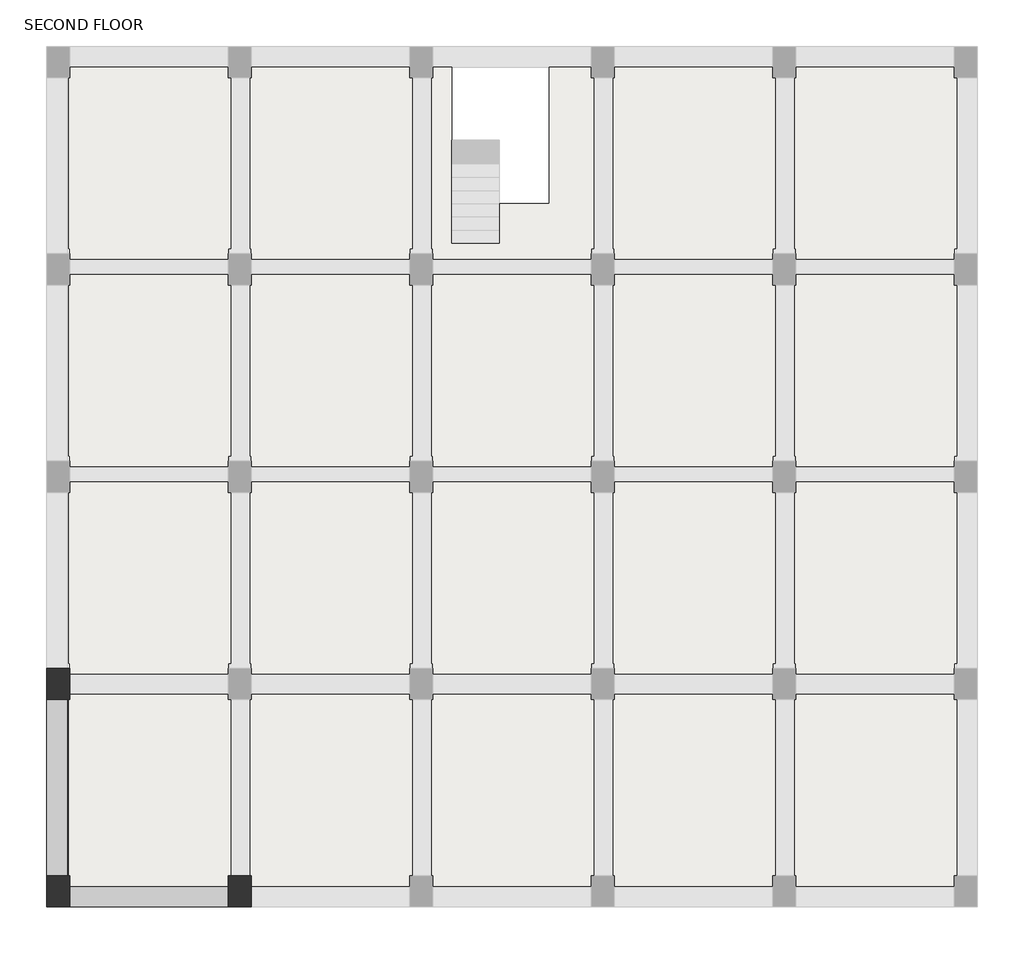
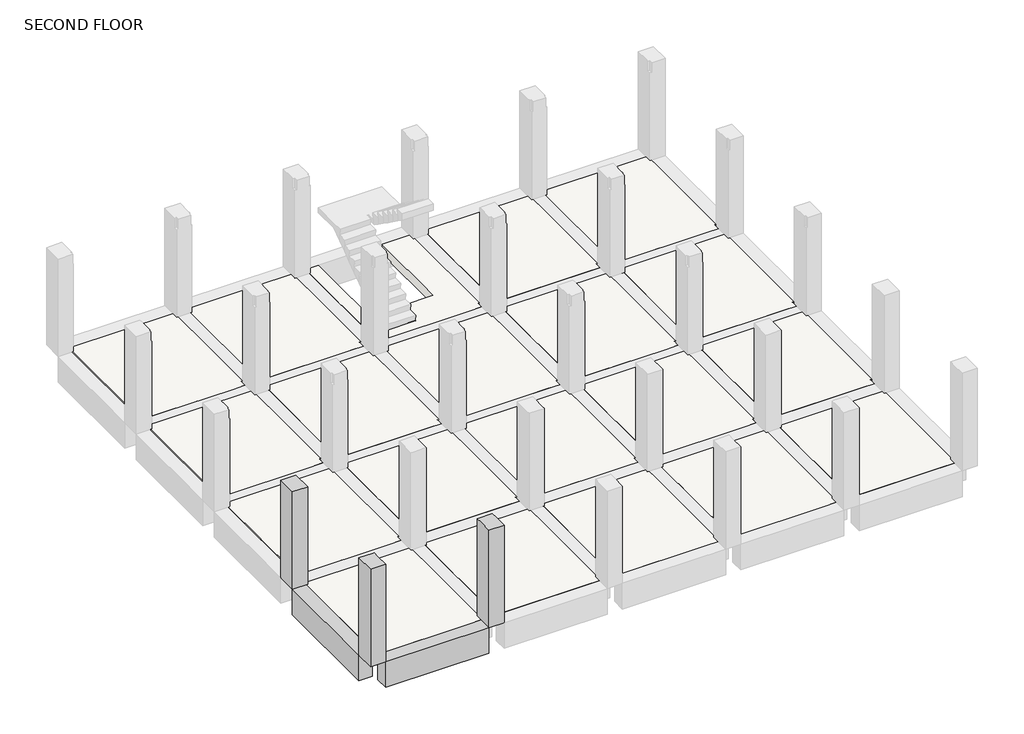
# One storey, part 1 of 3: 20 slabs, 3 columns, 2 beams.
"""IFC4 building model written with IfcOpenShell, lengths in millimetres."""

from ifc_helpers import new_model, si_unit, frame, origin, place, context, project, spatial, polyline, outline, extrude, faceted_brep, element, save

model = new_model("IFC4")

# Units and contexts
model_context = context("Model", 3, world=origin())
ifc_project = project(units=[si_unit("LENGTHUNIT", "METRE", prefix="MILLI")], contexts=[model_context])

# Site, building, storey
site = spatial("IfcSite", under=ifc_project)
building = spatial("IfcBuilding", under=site)
storey = spatial("IfcBuildingStorey", under=building, Name="SECOND FLOOR", Elevation=6096.0)

# Beams
placement = place(None, origin())
element("IfcBeam", 1, ObjectType="M_Concrete-Rectangular Beam : 400 x 800mm", at=placement, inside=storey, context=model_context, shape_type="Brep", body=[
    faceted_brep([(-9144.8884094, 3503.1212443, 6096.0), (-9144.8884094, 3103.1212443, 6096.0), (-6094.8884094, 3103.1212443, 6096.0), (-6094.8884094, 3503.1212443, 6096.0), (-9144.8884094, 3503.1212443, 5296.0), (-9144.8884094, 3503.1212443, 5796.0), (-6094.8884094, 3503.1212443, 5796.0), (-6094.8884094, 3503.1212443, 5296.0), (-9144.8884094, 3103.1212443, 5296.0), (-6094.8884094, 3103.1212443, 5296.0)], [[[0, 1, 2, 3]], [[4, 5, 0, 3, 6, 7]], [[8, 4, 7, 9]], [[1, 8, 9, 2]], [[1, 0, 5, 4, 8]], [[3, 2, 9, 7, 6]]]),
])
element("IfcBeam", 2, ObjectType="M_Concrete-Rectangular Beam : 400 x 800mm", at=placement, inside=storey, context=model_context, shape_type="SweptSolid", body=[
    extrude(outline(polyline([(-9594.8884094, 7103.1212443), (-9194.8884094, 7103.1212443), (-9194.8884094, 3703.1212443), (-9594.8884094, 3703.1212443), (-9594.8884094, 7103.1212443)])), frame((0.0, 0.0, 5296.0), z_axis=(0.0, 0.0, 1.0), x_axis=(1.0, 0.0, 0.0)), (0.0, 0.0, 1.0), 800.0),
])

# Columns
element("IfcColumn", 3, ObjectType="M_Concrete-Rectangular-Column : 450 x 600mm", at=placement, inside=storey, context=model_context, shape_type="Brep", body=[
    faceted_brep([(-9144.8884094, 7703.1212443, 6096.0), (-9144.8884094, 7103.1212443, 6096.0), (-9594.8884094, 7103.1212443, 6096.0), (-9594.8884094, 7703.1212443, 6096.0), (-9144.8884094, 7703.1212443, 8844.0), (-9144.8884094, 7703.1212443, 9144.0), (-9144.8884094, 7603.1212443, 9144.0), (-9144.8884094, 7203.1212443, 9144.0), (-9144.8884094, 7103.1212443, 9144.0), (-9144.8884094, 7103.1212443, 8844.0), (-9169.8884094, 7103.1212443, 9144.0), (-9594.8884094, 7103.1212443, 9144.0), (-9594.8884094, 7703.1212443, 9144.0)], [[[0, 1, 2, 3]], [[1, 0, 4, 5, 6, 7, 8, 9]], [[2, 1, 9, 8, 10, 11]], [[3, 2, 11, 12]], [[0, 3, 12, 5, 4]], [[12, 11, 10, 8, 7, 6, 5]]]),
])
element("IfcColumn", 4, ObjectType="M_Concrete-Rectangular-Column : 450 x 600mm", at=placement, inside=storey, context=model_context, shape_type="Brep", body=[
    faceted_brep([(-9144.8884094, 3703.1212443, 6096.0), (-9144.8884094, 3103.1212443, 6096.0), (-9594.8884094, 3103.1212443, 6096.0), (-9594.8884094, 3703.1212443, 6096.0), (-9144.8884094, 3703.1212443, 8844.0), (-9144.8884094, 3703.1212443, 9144.0), (-9144.8884094, 3503.1212443, 9144.0), (-9144.8884094, 3103.1212443, 9144.0), (-9594.8884094, 3103.1212443, 9144.0), (-9594.8884094, 3703.1212443, 9144.0), (-9169.8884094, 3703.1212443, 9144.0)], [[[0, 1, 2, 3]], [[1, 0, 4, 5, 6, 7]], [[2, 1, 7, 8]], [[3, 2, 8, 9]], [[0, 3, 9, 10, 5, 4]], [[8, 7, 6, 5, 10, 9]]]),
])
element("IfcColumn", 5, ObjectType="M_Concrete-Rectangular-Column : 450 x 600mm", at=placement, inside=storey, context=model_context, shape_type="Brep", body=[
    faceted_brep([(-5644.8884094, 3703.1212443, 6096.0), (-5644.8884094, 3103.1212443, 6096.0), (-6094.8884094, 3103.1212443, 6096.0), (-6094.8884094, 3703.1212443, 6096.0), (-5644.8884094, 3703.1212443, 8844.0), (-5644.8884094, 3703.1212443, 9144.0), (-5644.8884094, 3503.1212443, 9144.0), (-5644.8884094, 3103.1212443, 9144.0), (-6094.8884094, 3103.1212443, 9144.0), (-6094.8884094, 3503.1212443, 9144.0), (-6094.8884094, 3703.1212443, 9144.0), (-6094.8884094, 3703.1212443, 8844.0), (-6044.8884094, 3703.1212443, 9144.0), (-5669.8884094, 3703.1212443, 9144.0)], [[[0, 1, 2, 3]], [[1, 0, 4, 5, 6, 7]], [[2, 1, 7, 8]], [[3, 2, 8, 9, 10, 11]], [[0, 3, 11, 10, 12, 13, 5, 4]], [[8, 7, 6, 5, 13, 12, 10, 9]]]),
])

# Slabs
element("IfcSlab", 6, ObjectType="Generic 300mm", at=placement, inside=storey, context=model_context, shape_type="SweptSolid", body=[
    extrude(outline(polyline([(7955.1115906, 7103.1212443), (7955.1115906, 3703.1212443), (7905.1115906, 3703.1212443), (7905.1115906, 3503.1212443), (7530.1115906, 3503.1212443), (4855.1115906, 3503.1212443), (4855.1115906, 3703.1212443), (4830.1115906, 3703.1212443), (4830.1115906, 7103.1212443), (4855.1115906, 7103.1212443), (4855.1115906, 7203.1212443), (7905.1115906, 7203.1212443), (7905.1115906, 7103.1212443), (7955.1115906, 7103.1212443)])), frame((0.0, 0.0, 5796.0), z_axis=(0.0, 0.0, 1.0), x_axis=(1.0, 0.0, 0.0)), (0.0, 0.0, 1.0), 300.0),
])
element("IfcSlab", 7, ObjectType="Generic 300mm", at=placement, inside=storey, context=model_context, shape_type="Brep", body=[
    faceted_brep([(7955.1115906, 11203.1212443, 5796.0), (7955.1115906, 11103.1212443, 5796.0), (7955.1115906, 7803.1212443, 5796.0), (7905.1115906, 7803.1212443, 5796.0), (7905.1115906, 7603.1212443, 5796.0), (7530.1115906, 7603.1212443, 5796.0), (4855.1115906, 7603.1212443, 5796.0), (4855.1115906, 7803.1212443, 5796.0), (4830.1115906, 7803.1212443, 5796.0), (4830.1115906, 11103.1212443, 5796.0), (4830.1115906, 11203.1212443, 5796.0), (4855.1115906, 11203.1212443, 5796.0), (4855.1115906, 11303.1212443, 5796.0), (7905.1115906, 11303.1212443, 5796.0), (7905.1115906, 11203.1212443, 5796.0), (7955.1115906, 11203.1212443, 6096.0), (7905.1115906, 11203.1212443, 6096.0), (7905.1115906, 11303.1212443, 6096.0), (4855.1115906, 11303.1212443, 6096.0), (4855.1115906, 11203.1212443, 6096.0), (4830.1115906, 11203.1212443, 6096.0), (4830.1115906, 11103.1212443, 6096.0), (4830.1115906, 7803.1212443, 6096.0), (4855.1115906, 7803.1212443, 6096.0), (4855.1115906, 7703.1212443, 6096.0), (4855.1115906, 7603.1212443, 6096.0), (7530.1115906, 7603.1212443, 6096.0), (7905.1115906, 7603.1212443, 6096.0), (7905.1115906, 7703.1212443, 6096.0), (7905.1115906, 7803.1212443, 6096.0), (7955.1115906, 7803.1212443, 6096.0), (7955.1115906, 11103.1212443, 6096.0)], [[[0, 1, 2, 3, 4, 5, 6, 7, 8, 9, 10, 11, 12, 13, 14]], [[15, 16, 17, 18, 19, 20, 21, 22, 23, 24, 25, 26, 27, 28, 29, 30, 31]], [[2, 1, 0, 15, 31, 30]], [[3, 2, 30, 29]], [[4, 3, 29, 28, 27]], [[5, 4, 27, 26]], [[6, 5, 26, 25]], [[7, 6, 25, 24, 23]], [[8, 7, 23, 22]], [[10, 9, 8, 22, 21, 20]], [[11, 10, 20, 19]], [[12, 11, 19, 18]], [[13, 12, 18, 17]], [[14, 13, 17, 16]], [[0, 14, 16, 15]]]),
])
element("IfcSlab", 8, ObjectType="Generic 300mm", at=placement, inside=storey, context=model_context, shape_type="Brep", body=[
    faceted_brep([(4455.1115906, 11203.1212443, 5796.0), (4455.1115906, 11103.1212443, 5796.0), (4455.1115906, 7803.1212443, 5796.0), (4430.1115906, 7803.1212443, 5796.0), (4405.1115906, 7803.1212443, 5796.0), (4405.1115906, 7603.1212443, 5796.0), (4030.1115906, 7603.1212443, 5796.0), (1355.1115906, 7603.1212443, 5796.0), (1355.1115906, 7803.1212443, 5796.0), (1330.1115906, 7803.1212443, 5796.0), (1330.1115906, 11103.1212443, 5796.0), (1330.1115906, 11203.1212443, 5796.0), (1355.1115906, 11203.1212443, 5796.0), (1355.1115906, 11303.1212443, 5796.0), (4405.1115906, 11303.1212443, 5796.0), (4405.1115906, 11203.1212443, 5796.0), (4455.1115906, 11203.1212443, 6096.0), (4405.1115906, 11203.1212443, 6096.0), (4405.1115906, 11303.1212443, 6096.0), (1355.1115906, 11303.1212443, 6096.0), (1355.1115906, 11203.1212443, 6096.0), (1330.1115906, 11203.1212443, 6096.0), (1330.1115906, 11103.1212443, 6096.0), (1330.1115906, 7803.1212443, 6096.0), (1355.1115906, 7803.1212443, 6096.0), (1355.1115906, 7703.1212443, 6096.0), (1355.1115906, 7603.1212443, 6096.0), (4030.1115906, 7603.1212443, 6096.0), (4405.1115906, 7603.1212443, 6096.0), (4405.1115906, 7703.1212443, 6096.0), (4405.1115906, 7803.1212443, 6096.0), (4430.1115906, 7803.1212443, 6096.0), (4455.1115906, 7803.1212443, 6096.0), (4455.1115906, 11103.1212443, 6096.0)], [[[0, 1, 2, 3, 4, 5, 6, 7, 8, 9, 10, 11, 12, 13, 14, 15]], [[16, 17, 18, 19, 20, 21, 22, 23, 24, 25, 26, 27, 28, 29, 30, 31, 32, 33]], [[2, 1, 0, 16, 33, 32]], [[4, 3, 2, 32, 31, 30]], [[5, 4, 30, 29, 28]], [[6, 5, 28, 27]], [[7, 6, 27, 26]], [[8, 7, 26, 25, 24]], [[9, 8, 24, 23]], [[11, 10, 9, 23, 22, 21]], [[12, 11, 21, 20]], [[13, 12, 20, 19]], [[14, 13, 19, 18]], [[15, 14, 18, 17]], [[0, 15, 17, 16]]]),
])
element("IfcSlab", 9, ObjectType="Generic 300mm", at=placement, inside=storey, context=model_context, shape_type="Brep", body=[
    faceted_brep([(955.1115906, 11203.1212443, 5796.0), (955.1115906, 11103.1212443, 5796.0), (955.1115906, 7803.1212443, 5796.0), (930.1115906, 7803.1212443, 5796.0), (905.1115906, 7803.1212443, 5796.0), (905.1115906, 7603.1212443, 5796.0), (530.1115906, 7603.1212443, 5796.0), (-2144.8884094, 7603.1212443, 5796.0), (-2144.8884094, 7803.1212443, 5796.0), (-2169.8884094, 7803.1212443, 5796.0), (-2169.8884094, 11103.1212443, 5796.0), (-2169.8884094, 11203.1212443, 5796.0), (-2144.8884094, 11203.1212443, 5796.0), (-2144.8884094, 11303.1212443, 5796.0), (905.1115906, 11303.1212443, 5796.0), (905.1115906, 11203.1212443, 5796.0), (955.1115906, 11203.1212443, 6096.0), (905.1115906, 11203.1212443, 6096.0), (905.1115906, 11303.1212443, 6096.0), (-2144.8884094, 11303.1212443, 6096.0), (-2144.8884094, 11203.1212443, 6096.0), (-2169.8884094, 11203.1212443, 6096.0), (-2169.8884094, 11103.1212443, 6096.0), (-2169.8884094, 7803.1212443, 6096.0), (-2144.8884094, 7803.1212443, 6096.0), (-2144.8884094, 7703.1212443, 6096.0), (-2144.8884094, 7603.1212443, 6096.0), (530.1115906, 7603.1212443, 6096.0), (905.1115906, 7603.1212443, 6096.0), (905.1115906, 7703.1212443, 6096.0), (905.1115906, 7803.1212443, 6096.0), (930.1115906, 7803.1212443, 6096.0), (955.1115906, 7803.1212443, 6096.0), (955.1115906, 11103.1212443, 6096.0)], [[[0, 1, 2, 3, 4, 5, 6, 7, 8, 9, 10, 11, 12, 13, 14, 15]], [[16, 17, 18, 19, 20, 21, 22, 23, 24, 25, 26, 27, 28, 29, 30, 31, 32, 33]], [[2, 1, 0, 16, 33, 32]], [[4, 3, 2, 32, 31, 30]], [[5, 4, 30, 29, 28]], [[6, 5, 28, 27]], [[7, 6, 27, 26]], [[8, 7, 26, 25, 24]], [[9, 8, 24, 23]], [[11, 10, 9, 23, 22, 21]], [[12, 11, 21, 20]], [[13, 12, 20, 19]], [[14, 13, 19, 18]], [[15, 14, 18, 17]], [[0, 15, 17, 16]]]),
])
element("IfcSlab", 10, ObjectType="Generic 300mm", at=placement, inside=storey, context=model_context, shape_type="Brep", body=[
    faceted_brep([(-2544.8884094, 11203.1212443, 5796.0), (-2544.8884094, 11103.1212443, 5796.0), (-2544.8884094, 7803.1212443, 5796.0), (-2569.8884094, 7803.1212443, 5796.0), (-2594.8884094, 7803.1212443, 5796.0), (-2594.8884094, 7603.1212443, 5796.0), (-2969.8884094, 7603.1212443, 5796.0), (-5644.8884094, 7603.1212443, 5796.0), (-5644.8884094, 7803.1212443, 5796.0), (-5669.8884094, 7803.1212443, 5796.0), (-5669.8884094, 11103.1212443, 5796.0), (-5669.8884094, 11203.1212443, 5796.0), (-5644.8884094, 11203.1212443, 5796.0), (-5644.8884094, 11303.1212443, 5796.0), (-2594.8884094, 11303.1212443, 5796.0), (-2594.8884094, 11203.1212443, 5796.0), (-2544.8884094, 11203.1212443, 6096.0), (-2594.8884094, 11203.1212443, 6096.0), (-2594.8884094, 11303.1212443, 6096.0), (-5644.8884094, 11303.1212443, 6096.0), (-5644.8884094, 11203.1212443, 6096.0), (-5669.8884094, 11203.1212443, 6096.0), (-5669.8884094, 11103.1212443, 6096.0), (-5669.8884094, 7803.1212443, 6096.0), (-5644.8884094, 7803.1212443, 6096.0), (-5644.8884094, 7703.1212443, 6096.0), (-5644.8884094, 7603.1212443, 6096.0), (-2969.8884094, 7603.1212443, 6096.0), (-2594.8884094, 7603.1212443, 6096.0), (-2594.8884094, 7703.1212443, 6096.0), (-2594.8884094, 7803.1212443, 6096.0), (-2569.8884094, 7803.1212443, 6096.0), (-2544.8884094, 7803.1212443, 6096.0), (-2544.8884094, 11103.1212443, 6096.0)], [[[0, 1, 2, 3, 4, 5, 6, 7, 8, 9, 10, 11, 12, 13, 14, 15]], [[16, 17, 18, 19, 20, 21, 22, 23, 24, 25, 26, 27, 28, 29, 30, 31, 32, 33]], [[2, 1, 0, 16, 33, 32]], [[4, 3, 2, 32, 31, 30]], [[5, 4, 30, 29, 28]], [[6, 5, 28, 27]], [[7, 6, 27, 26]], [[8, 7, 26, 25, 24]], [[9, 8, 24, 23]], [[11, 10, 9, 23, 22, 21]], [[12, 11, 21, 20]], [[13, 12, 20, 19]], [[14, 13, 19, 18]], [[15, 14, 18, 17]], [[0, 15, 17, 16]]]),
])
element("IfcSlab", 11, ObjectType="Generic 300mm", at=placement, inside=storey, context=model_context, shape_type="Brep", body=[
    faceted_brep([(-6044.8884094, 11203.1212443, 5796.0), (-6044.8884094, 11103.1212443, 5796.0), (-6044.8884094, 7803.1212443, 5796.0), (-6069.8884094, 7803.1212443, 5796.0), (-6094.8884094, 7803.1212443, 5796.0), (-6094.8884094, 7603.1212443, 5796.0), (-6469.8884094, 7603.1212443, 5796.0), (-9144.8884094, 7603.1212443, 5796.0), (-9144.8884094, 7803.1212443, 5796.0), (-9169.8884094, 7803.1212443, 5796.0), (-9169.8884094, 11103.1212443, 5796.0), (-9169.8884094, 11203.1212443, 5796.0), (-9144.8884094, 11203.1212443, 5796.0), (-9144.8884094, 11303.1212443, 5796.0), (-6094.8884094, 11303.1212443, 5796.0), (-6094.8884094, 11203.1212443, 5796.0), (-6044.8884094, 11203.1212443, 6096.0), (-6094.8884094, 11203.1212443, 6096.0), (-6094.8884094, 11303.1212443, 6096.0), (-9144.8884094, 11303.1212443, 6096.0), (-9144.8884094, 11203.1212443, 6096.0), (-9169.8884094, 11203.1212443, 6096.0), (-9169.8884094, 11103.1212443, 6096.0), (-9169.8884094, 7803.1212443, 6096.0), (-9144.8884094, 7803.1212443, 6096.0), (-9144.8884094, 7703.1212443, 6096.0), (-9144.8884094, 7603.1212443, 6096.0), (-6469.8884094, 7603.1212443, 6096.0), (-6094.8884094, 7603.1212443, 6096.0), (-6094.8884094, 7703.1212443, 6096.0), (-6094.8884094, 7803.1212443, 6096.0), (-6069.8884094, 7803.1212443, 6096.0), (-6044.8884094, 7803.1212443, 6096.0), (-6044.8884094, 11103.1212443, 6096.0)], [[[0, 1, 2, 3, 4, 5, 6, 7, 8, 9, 10, 11, 12, 13, 14, 15]], [[16, 17, 18, 19, 20, 21, 22, 23, 24, 25, 26, 27, 28, 29, 30, 31, 32, 33]], [[2, 1, 0, 16, 33, 32]], [[4, 3, 2, 32, 31, 30]], [[5, 4, 30, 29, 28]], [[6, 5, 28, 27]], [[7, 6, 27, 26]], [[8, 7, 26, 25, 24]], [[9, 8, 24, 23]], [[11, 10, 9, 23, 22, 21]], [[12, 11, 21, 20]], [[13, 12, 20, 19]], [[14, 13, 19, 18]], [[15, 14, 18, 17]], [[0, 15, 17, 16]]]),
])
element("IfcSlab", 12, ObjectType="Generic 300mm", at=placement, inside=storey, context=model_context, shape_type="Brep", body=[
    faceted_brep([(-6044.8884094, 7103.1212443, 5796.0), (-6044.8884094, 3703.1212443, 5796.0), (-6069.8884094, 3703.1212443, 5796.0), (-6094.8884094, 3703.1212443, 5796.0), (-6094.8884094, 3503.1212443, 5796.0), (-6469.8884094, 3503.1212443, 5796.0), (-9144.8884094, 3503.1212443, 5796.0), (-9144.8884094, 3703.1212443, 5796.0), (-9169.8884094, 3703.1212443, 5796.0), (-9169.8884094, 7103.1212443, 5796.0), (-9144.8884094, 7103.1212443, 5796.0), (-9144.8884094, 7203.1212443, 5796.0), (-6094.8884094, 7203.1212443, 5796.0), (-6094.8884094, 7103.1212443, 5796.0), (-6069.8884094, 7103.1212443, 5796.0), (-6044.8884094, 7103.1212443, 6096.0), (-6094.8884094, 7103.1212443, 6096.0), (-6094.8884094, 7203.1212443, 6096.0), (-9144.8884094, 7203.1212443, 6096.0), (-9144.8884094, 7103.1212443, 6096.0), (-9169.8884094, 7103.1212443, 6096.0), (-9169.8884094, 3703.1212443, 6096.0), (-9144.8884094, 3703.1212443, 6096.0), (-9144.8884094, 3503.1212443, 6096.0), (-6469.8884094, 3503.1212443, 6096.0), (-6094.8884094, 3503.1212443, 6096.0), (-6094.8884094, 3703.1212443, 6096.0), (-6044.8884094, 3703.1212443, 6096.0)], [[[0, 1, 2, 3, 4, 5, 6, 7, 8, 9, 10, 11, 12, 13, 14]], [[15, 16, 17, 18, 19, 20, 21, 22, 23, 24, 25, 26, 27]], [[1, 0, 15, 27]], [[3, 2, 1, 27, 26]], [[4, 3, 26, 25]], [[5, 4, 25, 24]], [[6, 5, 24, 23]], [[7, 6, 23, 22]], [[8, 7, 22, 21]], [[9, 8, 21, 20]], [[10, 9, 20, 19]], [[11, 10, 19, 18]], [[12, 11, 18, 17]], [[13, 12, 17, 16]], [[0, 14, 13, 16, 15]]]),
])
element("IfcSlab", 13, ObjectType="Generic 300mm", at=placement, inside=storey, context=model_context, shape_type="Brep", body=[
    faceted_brep([(-2544.8884094, 7103.1212443, 5796.0), (-2544.8884094, 3703.1212443, 5796.0), (-2569.8884094, 3703.1212443, 5796.0), (-2594.8884094, 3703.1212443, 5796.0), (-2594.8884094, 3503.1212443, 5796.0), (-2969.8884094, 3503.1212443, 5796.0), (-5644.8884094, 3503.1212443, 5796.0), (-5644.8884094, 3703.1212443, 5796.0), (-5669.8884094, 3703.1212443, 5796.0), (-5669.8884094, 7103.1212443, 5796.0), (-5644.8884094, 7103.1212443, 5796.0), (-5644.8884094, 7203.1212443, 5796.0), (-2594.8884094, 7203.1212443, 5796.0), (-2594.8884094, 7103.1212443, 5796.0), (-2569.8884094, 7103.1212443, 5796.0), (-2544.8884094, 7103.1212443, 6096.0), (-2594.8884094, 7103.1212443, 6096.0), (-2594.8884094, 7203.1212443, 6096.0), (-5644.8884094, 7203.1212443, 6096.0), (-5644.8884094, 7103.1212443, 6096.0), (-5669.8884094, 7103.1212443, 6096.0), (-5669.8884094, 3703.1212443, 6096.0), (-5644.8884094, 3703.1212443, 6096.0), (-5644.8884094, 3503.1212443, 6096.0), (-2969.8884094, 3503.1212443, 6096.0), (-2594.8884094, 3503.1212443, 6096.0), (-2594.8884094, 3703.1212443, 6096.0), (-2544.8884094, 3703.1212443, 6096.0)], [[[0, 1, 2, 3, 4, 5, 6, 7, 8, 9, 10, 11, 12, 13, 14]], [[15, 16, 17, 18, 19, 20, 21, 22, 23, 24, 25, 26, 27]], [[1, 0, 15, 27]], [[3, 2, 1, 27, 26]], [[4, 3, 26, 25]], [[5, 4, 25, 24]], [[6, 5, 24, 23]], [[7, 6, 23, 22]], [[8, 7, 22, 21]], [[9, 8, 21, 20]], [[10, 9, 20, 19]], [[11, 10, 19, 18]], [[12, 11, 18, 17]], [[13, 12, 17, 16]], [[0, 14, 13, 16, 15]]]),
])
element("IfcSlab", 14, ObjectType="Generic 300mm", at=placement, inside=storey, context=model_context, shape_type="Brep", body=[
    faceted_brep([(955.1115906, 7103.1212443, 5796.0), (955.1115906, 3703.1212443, 5796.0), (930.1115906, 3703.1212443, 5796.0), (905.1115906, 3703.1212443, 5796.0), (905.1115906, 3503.1212443, 5796.0), (530.1115906, 3503.1212443, 5796.0), (-2144.8884094, 3503.1212443, 5796.0), (-2144.8884094, 3703.1212443, 5796.0), (-2169.8884094, 3703.1212443, 5796.0), (-2169.8884094, 7103.1212443, 5796.0), (-2144.8884094, 7103.1212443, 5796.0), (-2144.8884094, 7203.1212443, 5796.0), (905.1115906, 7203.1212443, 5796.0), (905.1115906, 7103.1212443, 5796.0), (930.1115906, 7103.1212443, 5796.0), (955.1115906, 7103.1212443, 6096.0), (905.1115906, 7103.1212443, 6096.0), (905.1115906, 7203.1212443, 6096.0), (-2144.8884094, 7203.1212443, 6096.0), (-2144.8884094, 7103.1212443, 6096.0), (-2169.8884094, 7103.1212443, 6096.0), (-2169.8884094, 3703.1212443, 6096.0), (-2144.8884094, 3703.1212443, 6096.0), (-2144.8884094, 3503.1212443, 6096.0), (530.1115906, 3503.1212443, 6096.0), (905.1115906, 3503.1212443, 6096.0), (905.1115906, 3703.1212443, 6096.0), (955.1115906, 3703.1212443, 6096.0)], [[[0, 1, 2, 3, 4, 5, 6, 7, 8, 9, 10, 11, 12, 13, 14]], [[15, 16, 17, 18, 19, 20, 21, 22, 23, 24, 25, 26, 27]], [[1, 0, 15, 27]], [[3, 2, 1, 27, 26]], [[4, 3, 26, 25]], [[5, 4, 25, 24]], [[6, 5, 24, 23]], [[7, 6, 23, 22]], [[8, 7, 22, 21]], [[9, 8, 21, 20]], [[10, 9, 20, 19]], [[11, 10, 19, 18]], [[12, 11, 18, 17]], [[13, 12, 17, 16]], [[0, 14, 13, 16, 15]]]),
])
element("IfcSlab", 15, ObjectType="Generic 300mm", at=placement, inside=storey, context=model_context, shape_type="Brep", body=[
    faceted_brep([(4455.1115906, 7103.1212443, 5796.0), (4455.1115906, 3703.1212443, 5796.0), (4430.1115906, 3703.1212443, 5796.0), (4405.1115906, 3703.1212443, 5796.0), (4405.1115906, 3503.1212443, 5796.0), (4030.1115906, 3503.1212443, 5796.0), (1355.1115906, 3503.1212443, 5796.0), (1355.1115906, 3703.1212443, 5796.0), (1330.1115906, 3703.1212443, 5796.0), (1330.1115906, 7103.1212443, 5796.0), (1355.1115906, 7103.1212443, 5796.0), (1355.1115906, 7203.1212443, 5796.0), (4405.1115906, 7203.1212443, 5796.0), (4405.1115906, 7103.1212443, 5796.0), (4430.1115906, 7103.1212443, 5796.0), (4455.1115906, 7103.1212443, 6096.0), (4405.1115906, 7103.1212443, 6096.0), (4405.1115906, 7203.1212443, 6096.0), (1355.1115906, 7203.1212443, 6096.0), (1355.1115906, 7103.1212443, 6096.0), (1330.1115906, 7103.1212443, 6096.0), (1330.1115906, 3703.1212443, 6096.0), (1355.1115906, 3703.1212443, 6096.0), (1355.1115906, 3503.1212443, 6096.0), (4030.1115906, 3503.1212443, 6096.0), (4405.1115906, 3503.1212443, 6096.0), (4405.1115906, 3703.1212443, 6096.0), (4455.1115906, 3703.1212443, 6096.0)], [[[0, 1, 2, 3, 4, 5, 6, 7, 8, 9, 10, 11, 12, 13, 14]], [[15, 16, 17, 18, 19, 20, 21, 22, 23, 24, 25, 26, 27]], [[1, 0, 15, 27]], [[3, 2, 1, 27, 26]], [[4, 3, 26, 25]], [[5, 4, 25, 24]], [[6, 5, 24, 23]], [[7, 6, 23, 22]], [[8, 7, 22, 21]], [[9, 8, 21, 20]], [[10, 9, 20, 19]], [[11, 10, 19, 18]], [[12, 11, 18, 17]], [[13, 12, 17, 16]], [[0, 14, 13, 16, 15]]]),
])
element("IfcSlab", 16, ObjectType="Generic 300mm", at=placement, inside=storey, context=model_context, shape_type="Brep", body=[
    faceted_brep([(7955.1115906, 15203.1212443, 5796.0), (7955.1115906, 15103.1212443, 5796.0), (7955.1115906, 11803.1212443, 5796.0), (7905.1115906, 11803.1212443, 5796.0), (7905.1115906, 11603.1212443, 5796.0), (7530.1115906, 11603.1212443, 5796.0), (4855.1115906, 11603.1212443, 5796.0), (4855.1115906, 11803.1212443, 5796.0), (4830.1115906, 11803.1212443, 5796.0), (4830.1115906, 15103.1212443, 5796.0), (4830.1115906, 15203.1212443, 5796.0), (4855.1115906, 15203.1212443, 5796.0), (4855.1115906, 15303.1212443, 5796.0), (7905.1115906, 15303.1212443, 5796.0), (7905.1115906, 15203.1212443, 5796.0), (7955.1115906, 15203.1212443, 6096.0), (7905.1115906, 15203.1212443, 6096.0), (7905.1115906, 15303.1212443, 6096.0), (4855.1115906, 15303.1212443, 6096.0), (4855.1115906, 15203.1212443, 6096.0), (4830.1115906, 15203.1212443, 6096.0), (4830.1115906, 15103.1212443, 6096.0), (4830.1115906, 11803.1212443, 6096.0), (4855.1115906, 11803.1212443, 6096.0), (4855.1115906, 11703.1212443, 6096.0), (4855.1115906, 11603.1212443, 6096.0), (7530.1115906, 11603.1212443, 6096.0), (7905.1115906, 11603.1212443, 6096.0), (7905.1115906, 11703.1212443, 6096.0), (7905.1115906, 11803.1212443, 6096.0), (7955.1115906, 11803.1212443, 6096.0), (7955.1115906, 15103.1212443, 6096.0)], [[[0, 1, 2, 3, 4, 5, 6, 7, 8, 9, 10, 11, 12, 13, 14]], [[15, 16, 17, 18, 19, 20, 21, 22, 23, 24, 25, 26, 27, 28, 29, 30, 31]], [[2, 1, 0, 15, 31, 30]], [[3, 2, 30, 29]], [[4, 3, 29, 28, 27]], [[5, 4, 27, 26]], [[6, 5, 26, 25]], [[7, 6, 25, 24, 23]], [[8, 7, 23, 22]], [[10, 9, 8, 22, 21, 20]], [[11, 10, 20, 19]], [[12, 11, 19, 18]], [[13, 12, 18, 17]], [[14, 13, 17, 16]], [[0, 14, 16, 15]]]),
])
element("IfcSlab", 17, ObjectType="Generic 300mm", at=placement, inside=storey, context=model_context, shape_type="Brep", body=[
    faceted_brep([(7955.1115906, 19203.1212443, 5796.0), (7955.1115906, 19103.1212443, 5796.0), (7955.1115906, 15803.1212443, 5796.0), (7905.1115906, 15803.1212443, 5796.0), (7905.1115906, 15603.1212443, 5796.0), (7530.1115906, 15603.1212443, 5796.0), (4855.1115906, 15603.1212443, 5796.0), (4855.1115906, 15803.1212443, 5796.0), (4830.1115906, 15803.1212443, 5796.0), (4830.1115906, 19103.1212443, 5796.0), (4830.1115906, 19203.1212443, 5796.0), (4855.1115906, 19203.1212443, 5796.0), (4855.1115906, 19303.1212443, 5796.0), (7905.1115906, 19303.1212443, 5796.0), (7905.1115906, 19203.1212443, 5796.0), (7955.1115906, 19203.1212443, 6096.0), (7905.1115906, 19203.1212443, 6096.0), (7905.1115906, 19303.1212443, 6096.0), (4855.1115906, 19303.1212443, 6096.0), (4855.1115906, 19203.1212443, 6096.0), (4830.1115906, 19203.1212443, 6096.0), (4830.1115906, 19103.1212443, 6096.0), (4830.1115906, 15803.1212443, 6096.0), (4855.1115906, 15803.1212443, 6096.0), (4855.1115906, 15703.1212443, 6096.0), (4855.1115906, 15603.1212443, 6096.0), (7530.1115906, 15603.1212443, 6096.0), (7905.1115906, 15603.1212443, 6096.0), (7905.1115906, 15703.1212443, 6096.0), (7905.1115906, 15803.1212443, 6096.0), (7955.1115906, 15803.1212443, 6096.0), (7955.1115906, 19103.1212443, 6096.0)], [[[0, 1, 2, 3, 4, 5, 6, 7, 8, 9, 10, 11, 12, 13, 14]], [[15, 16, 17, 18, 19, 20, 21, 22, 23, 24, 25, 26, 27, 28, 29, 30, 31]], [[2, 1, 0, 15, 31, 30]], [[3, 2, 30, 29]], [[4, 3, 29, 28, 27]], [[5, 4, 27, 26]], [[6, 5, 26, 25]], [[7, 6, 25, 24, 23]], [[8, 7, 23, 22]], [[10, 9, 8, 22, 21, 20]], [[11, 10, 20, 19]], [[12, 11, 19, 18]], [[13, 12, 18, 17]], [[14, 13, 17, 16]], [[0, 14, 16, 15]]]),
])
element("IfcSlab", 18, ObjectType="Generic 300mm", at=placement, inside=storey, context=model_context, shape_type="Brep", body=[
    faceted_brep([(4455.1115906, 19203.1212443, 5796.0), (4455.1115906, 19103.1212443, 5796.0), (4455.1115906, 15803.1212443, 5796.0), (4430.1115906, 15803.1212443, 5796.0), (4405.1115906, 15803.1212443, 5796.0), (4405.1115906, 15603.1212443, 5796.0), (4030.1115906, 15603.1212443, 5796.0), (1355.1115906, 15603.1212443, 5796.0), (1355.1115906, 15803.1212443, 5796.0), (1330.1115906, 15803.1212443, 5796.0), (1330.1115906, 19103.1212443, 5796.0), (1330.1115906, 19203.1212443, 5796.0), (1355.1115906, 19203.1212443, 5796.0), (1355.1115906, 19303.1212443, 5796.0), (4405.1115906, 19303.1212443, 5796.0), (4405.1115906, 19203.1212443, 5796.0), (4455.1115906, 19203.1212443, 6096.0), (4405.1115906, 19203.1212443, 6096.0), (4405.1115906, 19303.1212443, 6096.0), (1355.1115906, 19303.1212443, 6096.0), (1355.1115906, 19203.1212443, 6096.0), (1330.1115906, 19203.1212443, 6096.0), (1330.1115906, 19103.1212443, 6096.0), (1330.1115906, 15803.1212443, 6096.0), (1355.1115906, 15803.1212443, 6096.0), (1355.1115906, 15703.1212443, 6096.0), (1355.1115906, 15603.1212443, 6096.0), (4030.1115906, 15603.1212443, 6096.0), (4405.1115906, 15603.1212443, 6096.0), (4405.1115906, 15703.1212443, 6096.0), (4405.1115906, 15803.1212443, 6096.0), (4430.1115906, 15803.1212443, 6096.0), (4455.1115906, 15803.1212443, 6096.0), (4455.1115906, 19103.1212443, 6096.0)], [[[0, 1, 2, 3, 4, 5, 6, 7, 8, 9, 10, 11, 12, 13, 14, 15]], [[16, 17, 18, 19, 20, 21, 22, 23, 24, 25, 26, 27, 28, 29, 30, 31, 32, 33]], [[2, 1, 0, 16, 33, 32]], [[4, 3, 2, 32, 31, 30]], [[5, 4, 30, 29, 28]], [[6, 5, 28, 27]], [[7, 6, 27, 26]], [[8, 7, 26, 25, 24]], [[9, 8, 24, 23]], [[11, 10, 9, 23, 22, 21]], [[12, 11, 21, 20]], [[13, 12, 20, 19]], [[14, 13, 19, 18]], [[15, 14, 18, 17]], [[0, 15, 17, 16]]]),
])
element("IfcSlab", 19, ObjectType="Generic 300mm", at=placement, inside=storey, context=model_context, shape_type="Brep", body=[
    faceted_brep([(4455.1115906, 15203.1212443, 5796.0), (4455.1115906, 15103.1212443, 5796.0), (4455.1115906, 11803.1212443, 5796.0), (4430.1115906, 11803.1212443, 5796.0), (4405.1115906, 11803.1212443, 5796.0), (4405.1115906, 11603.1212443, 5796.0), (4030.1115906, 11603.1212443, 5796.0), (1355.1115906, 11603.1212443, 5796.0), (1355.1115906, 11803.1212443, 5796.0), (1330.1115906, 11803.1212443, 5796.0), (1330.1115906, 15103.1212443, 5796.0), (1330.1115906, 15203.1212443, 5796.0), (1355.1115906, 15203.1212443, 5796.0), (1355.1115906, 15303.1212443, 5796.0), (4405.1115906, 15303.1212443, 5796.0), (4405.1115906, 15203.1212443, 5796.0), (4455.1115906, 15203.1212443, 6096.0), (4405.1115906, 15203.1212443, 6096.0), (4405.1115906, 15303.1212443, 6096.0), (1355.1115906, 15303.1212443, 6096.0), (1355.1115906, 15203.1212443, 6096.0), (1330.1115906, 15203.1212443, 6096.0), (1330.1115906, 15103.1212443, 6096.0), (1330.1115906, 11803.1212443, 6096.0), (1355.1115906, 11803.1212443, 6096.0), (1355.1115906, 11703.1212443, 6096.0), (1355.1115906, 11603.1212443, 6096.0), (4030.1115906, 11603.1212443, 6096.0), (4405.1115906, 11603.1212443, 6096.0), (4405.1115906, 11703.1212443, 6096.0), (4405.1115906, 11803.1212443, 6096.0), (4430.1115906, 11803.1212443, 6096.0), (4455.1115906, 11803.1212443, 6096.0), (4455.1115906, 15103.1212443, 6096.0)], [[[0, 1, 2, 3, 4, 5, 6, 7, 8, 9, 10, 11, 12, 13, 14, 15]], [[16, 17, 18, 19, 20, 21, 22, 23, 24, 25, 26, 27, 28, 29, 30, 31, 32, 33]], [[2, 1, 0, 16, 33, 32]], [[4, 3, 2, 32, 31, 30]], [[5, 4, 30, 29, 28]], [[6, 5, 28, 27]], [[7, 6, 27, 26]], [[8, 7, 26, 25, 24]], [[9, 8, 24, 23]], [[11, 10, 9, 23, 22, 21]], [[12, 11, 21, 20]], [[13, 12, 20, 19]], [[14, 13, 19, 18]], [[15, 14, 18, 17]], [[0, 15, 17, 16]]]),
])
element("IfcSlab", 20, ObjectType="Generic 300mm", at=placement, inside=storey, context=model_context, shape_type="Brep", body=[
    faceted_brep([(955.1115906, 15203.1212443, 5796.0), (955.1115906, 15103.1212443, 5796.0), (955.1115906, 11803.1212443, 5796.0), (930.1115906, 11803.1212443, 5796.0), (905.1115906, 11803.1212443, 5796.0), (905.1115906, 11603.1212443, 5796.0), (530.1115906, 11603.1212443, 5796.0), (-2144.8884094, 11603.1212443, 5796.0), (-2144.8884094, 11803.1212443, 5796.0), (-2169.8884094, 11803.1212443, 5796.0), (-2169.8884094, 15103.1212443, 5796.0), (-2169.8884094, 15203.1212443, 5796.0), (-2144.8884094, 15203.1212443, 5796.0), (-2144.8884094, 15303.1212443, 5796.0), (905.1115906, 15303.1212443, 5796.0), (905.1115906, 15203.1212443, 5796.0), (955.1115906, 15203.1212443, 6096.0), (905.1115906, 15203.1212443, 6096.0), (905.1115906, 15303.1212443, 6096.0), (-2144.8884094, 15303.1212443, 6096.0), (-2144.8884094, 15203.1212443, 6096.0), (-2169.8884094, 15203.1212443, 6096.0), (-2169.8884094, 15103.1212443, 6096.0), (-2169.8884094, 11803.1212443, 6096.0), (-2144.8884094, 11803.1212443, 6096.0), (-2144.8884094, 11703.1212443, 6096.0), (-2144.8884094, 11603.1212443, 6096.0), (530.1115906, 11603.1212443, 6096.0), (905.1115906, 11603.1212443, 6096.0), (905.1115906, 11703.1212443, 6096.0), (905.1115906, 11803.1212443, 6096.0), (930.1115906, 11803.1212443, 6096.0), (955.1115906, 11803.1212443, 6096.0), (955.1115906, 15103.1212443, 6096.0)], [[[0, 1, 2, 3, 4, 5, 6, 7, 8, 9, 10, 11, 12, 13, 14, 15]], [[16, 17, 18, 19, 20, 21, 22, 23, 24, 25, 26, 27, 28, 29, 30, 31, 32, 33]], [[2, 1, 0, 16, 33, 32]], [[4, 3, 2, 32, 31, 30]], [[5, 4, 30, 29, 28]], [[6, 5, 28, 27]], [[7, 6, 27, 26]], [[8, 7, 26, 25, 24]], [[9, 8, 24, 23]], [[11, 10, 9, 23, 22, 21]], [[12, 11, 21, 20]], [[13, 12, 20, 19]], [[14, 13, 19, 18]], [[15, 14, 18, 17]], [[0, 15, 17, 16]]]),
])
element("IfcSlab", 21, ObjectType="Generic 300mm", at=placement, inside=storey, context=model_context, shape_type="Brep", body=[
    faceted_brep([(955.1115906, 19203.1212443, 5796.0), (955.1115906, 19103.1212443, 5796.0), (955.1115906, 15803.1212443, 5796.0), (930.1115906, 15803.1212443, 5796.0), (905.1115906, 15803.1212443, 5796.0), (905.1115906, 15603.1212443, 5796.0), (530.1115906, 15603.1212443, 5796.0), (-2144.8884094, 15603.1212443, 5796.0), (-2144.8884094, 15803.1212443, 5796.0), (-2169.8884094, 15803.1212443, 5796.0), (-2169.8884094, 19103.1212443, 5796.0), (-2169.8884094, 19203.1212443, 5796.0), (-2144.8884094, 19203.1212443, 5796.0), (-2144.8884094, 19303.1212443, 5796.0), (-1784.8884094, 19303.1212443, 5796.0), (-1784.8884094, 15908.7212443, 5796.0), (-870.4884094, 15908.7212443, 5796.0), (-870.4884094, 16670.7212443, 5796.0), (-819.6884094, 16670.7212443, 5796.0), (94.7115906, 16670.7212443, 5796.0), (94.7115906, 19303.1212443, 5796.0), (905.1115906, 19303.1212443, 5796.0), (905.1115906, 19203.1212443, 5796.0), (955.1115906, 15803.1212443, 6096.0), (955.1115906, 19103.1212443, 6096.0), (955.1115906, 19203.1212443, 6096.0), (905.1115906, 19203.1212443, 6096.0), (905.1115906, 19303.1212443, 6096.0), (94.7115906, 19303.1212443, 6096.0), (94.7115906, 16670.7212443, 6096.0), (-819.6884094, 16670.7212443, 6096.0), (-870.4884094, 16670.7212443, 6096.0), (-870.4884094, 15908.7212443, 6096.0), (-1784.8884094, 15908.7212443, 6096.0), (-1784.8884094, 19303.1212443, 6096.0), (-2144.8884094, 19303.1212443, 6096.0), (-2144.8884094, 19203.1212443, 6096.0), (-2169.8884094, 19203.1212443, 6096.0), (-2169.8884094, 19103.1212443, 6096.0), (-2169.8884094, 15803.1212443, 6096.0), (-2144.8884094, 15803.1212443, 6096.0), (-2144.8884094, 15703.1212443, 6096.0), (-2144.8884094, 15603.1212443, 6096.0), (530.1115906, 15603.1212443, 6096.0), (905.1115906, 15603.1212443, 6096.0), (905.1115906, 15703.1212443, 6096.0), (905.1115906, 15803.1212443, 6096.0), (930.1115906, 15803.1212443, 6096.0)], [[[0, 1, 2, 3, 4, 5, 6, 7, 8, 9, 10, 11, 12, 13, 14, 15, 16, 17, 18, 19, 20, 21, 22]], [[23, 24, 25, 26, 27, 28, 29, 30, 31, 32, 33, 34, 35, 36, 37, 38, 39, 40, 41, 42, 43, 44, 45, 46, 47]], [[2, 1, 0, 25, 24, 23]], [[4, 3, 2, 23, 47, 46]], [[5, 4, 46, 45, 44]], [[6, 5, 44, 43]], [[7, 6, 43, 42]], [[8, 7, 42, 41, 40]], [[9, 8, 40, 39]], [[11, 10, 9, 39, 38, 37]], [[12, 11, 37, 36]], [[13, 12, 36, 35]], [[13, 35, 34, 14]], [[27, 21, 20, 28]], [[22, 21, 27, 26]], [[0, 22, 26, 25]], [[19, 29, 28, 20]], [[33, 15, 14, 34]], [[15, 33, 32, 16]], [[16, 32, 31, 17]], [[17, 31, 30, 18]], [[29, 19, 18, 30]]]),
])
element("IfcSlab", 22, ObjectType="Generic 300mm", at=placement, inside=storey, context=model_context, shape_type="Brep", body=[
    faceted_brep([(-2544.8884094, 19203.1212443, 5796.0), (-2544.8884094, 19103.1212443, 5796.0), (-2544.8884094, 15803.1212443, 5796.0), (-2569.8884094, 15803.1212443, 5796.0), (-2594.8884094, 15803.1212443, 5796.0), (-2594.8884094, 15603.1212443, 5796.0), (-2969.8884094, 15603.1212443, 5796.0), (-5644.8884094, 15603.1212443, 5796.0), (-5644.8884094, 15803.1212443, 5796.0), (-5669.8884094, 15803.1212443, 5796.0), (-5669.8884094, 19103.1212443, 5796.0), (-5669.8884094, 19203.1212443, 5796.0), (-5644.8884094, 19203.1212443, 5796.0), (-5644.8884094, 19303.1212443, 5796.0), (-2594.8884094, 19303.1212443, 5796.0), (-2594.8884094, 19203.1212443, 5796.0), (-2544.8884094, 19203.1212443, 6096.0), (-2594.8884094, 19203.1212443, 6096.0), (-2594.8884094, 19303.1212443, 6096.0), (-5644.8884094, 19303.1212443, 6096.0), (-5644.8884094, 19203.1212443, 6096.0), (-5669.8884094, 19203.1212443, 6096.0), (-5669.8884094, 19103.1212443, 6096.0), (-5669.8884094, 15803.1212443, 6096.0), (-5644.8884094, 15803.1212443, 6096.0), (-5644.8884094, 15703.1212443, 6096.0), (-5644.8884094, 15603.1212443, 6096.0), (-2969.8884094, 15603.1212443, 6096.0), (-2594.8884094, 15603.1212443, 6096.0), (-2594.8884094, 15703.1212443, 6096.0), (-2594.8884094, 15803.1212443, 6096.0), (-2569.8884094, 15803.1212443, 6096.0), (-2544.8884094, 15803.1212443, 6096.0), (-2544.8884094, 19103.1212443, 6096.0)], [[[0, 1, 2, 3, 4, 5, 6, 7, 8, 9, 10, 11, 12, 13, 14, 15]], [[16, 17, 18, 19, 20, 21, 22, 23, 24, 25, 26, 27, 28, 29, 30, 31, 32, 33]], [[2, 1, 0, 16, 33, 32]], [[4, 3, 2, 32, 31, 30]], [[5, 4, 30, 29, 28]], [[6, 5, 28, 27]], [[7, 6, 27, 26]], [[8, 7, 26, 25, 24]], [[9, 8, 24, 23]], [[11, 10, 9, 23, 22, 21]], [[12, 11, 21, 20]], [[13, 12, 20, 19]], [[14, 13, 19, 18]], [[15, 14, 18, 17]], [[0, 15, 17, 16]]]),
])
element("IfcSlab", 23, ObjectType="Generic 300mm", at=placement, inside=storey, context=model_context, shape_type="Brep", body=[
    faceted_brep([(-6044.8884094, 19203.1212443, 5796.0), (-6044.8884094, 19103.1212443, 5796.0), (-6044.8884094, 15803.1212443, 5796.0), (-6069.8884094, 15803.1212443, 5796.0), (-6094.8884094, 15803.1212443, 5796.0), (-6094.8884094, 15603.1212443, 5796.0), (-6469.8884094, 15603.1212443, 5796.0), (-9144.8884094, 15603.1212443, 5796.0), (-9144.8884094, 15803.1212443, 5796.0), (-9169.8884094, 15803.1212443, 5796.0), (-9169.8884094, 19103.1212443, 5796.0), (-9169.8884094, 19203.1212443, 5796.0), (-9144.8884094, 19203.1212443, 5796.0), (-9144.8884094, 19303.1212443, 5796.0), (-6094.8884094, 19303.1212443, 5796.0), (-6094.8884094, 19203.1212443, 5796.0), (-6044.8884094, 19203.1212443, 6096.0), (-6094.8884094, 19203.1212443, 6096.0), (-6094.8884094, 19303.1212443, 6096.0), (-9144.8884094, 19303.1212443, 6096.0), (-9144.8884094, 19203.1212443, 6096.0), (-9169.8884094, 19203.1212443, 6096.0), (-9169.8884094, 19103.1212443, 6096.0), (-9169.8884094, 15803.1212443, 6096.0), (-9144.8884094, 15803.1212443, 6096.0), (-9144.8884094, 15703.1212443, 6096.0), (-9144.8884094, 15603.1212443, 6096.0), (-6469.8884094, 15603.1212443, 6096.0), (-6094.8884094, 15603.1212443, 6096.0), (-6094.8884094, 15703.1212443, 6096.0), (-6094.8884094, 15803.1212443, 6096.0), (-6069.8884094, 15803.1212443, 6096.0), (-6044.8884094, 15803.1212443, 6096.0), (-6044.8884094, 19103.1212443, 6096.0)], [[[0, 1, 2, 3, 4, 5, 6, 7, 8, 9, 10, 11, 12, 13, 14, 15]], [[16, 17, 18, 19, 20, 21, 22, 23, 24, 25, 26, 27, 28, 29, 30, 31, 32, 33]], [[2, 1, 0, 16, 33, 32]], [[4, 3, 2, 32, 31, 30]], [[5, 4, 30, 29, 28]], [[6, 5, 28, 27]], [[7, 6, 27, 26]], [[8, 7, 26, 25, 24]], [[9, 8, 24, 23]], [[11, 10, 9, 23, 22, 21]], [[12, 11, 21, 20]], [[13, 12, 20, 19]], [[14, 13, 19, 18]], [[15, 14, 18, 17]], [[0, 15, 17, 16]]]),
])
element("IfcSlab", 24, ObjectType="Generic 300mm", at=placement, inside=storey, context=model_context, shape_type="Brep", body=[
    faceted_brep([(-6044.8884094, 15203.1212443, 5796.0), (-6044.8884094, 15103.1212443, 5796.0), (-6044.8884094, 11803.1212443, 5796.0), (-6069.8884094, 11803.1212443, 5796.0), (-6094.8884094, 11803.1212443, 5796.0), (-6094.8884094, 11603.1212443, 5796.0), (-6469.8884094, 11603.1212443, 5796.0), (-9144.8884094, 11603.1212443, 5796.0), (-9144.8884094, 11803.1212443, 5796.0), (-9169.8884094, 11803.1212443, 5796.0), (-9169.8884094, 15103.1212443, 5796.0), (-9169.8884094, 15203.1212443, 5796.0), (-9144.8884094, 15203.1212443, 5796.0), (-9144.8884094, 15303.1212443, 5796.0), (-6094.8884094, 15303.1212443, 5796.0), (-6094.8884094, 15203.1212443, 5796.0), (-6044.8884094, 15203.1212443, 6096.0), (-6094.8884094, 15203.1212443, 6096.0), (-6094.8884094, 15303.1212443, 6096.0), (-9144.8884094, 15303.1212443, 6096.0), (-9144.8884094, 15203.1212443, 6096.0), (-9169.8884094, 15203.1212443, 6096.0), (-9169.8884094, 15103.1212443, 6096.0), (-9169.8884094, 11803.1212443, 6096.0), (-9144.8884094, 11803.1212443, 6096.0), (-9144.8884094, 11703.1212443, 6096.0), (-9144.8884094, 11603.1212443, 6096.0), (-6469.8884094, 11603.1212443, 6096.0), (-6094.8884094, 11603.1212443, 6096.0), (-6094.8884094, 11703.1212443, 6096.0), (-6094.8884094, 11803.1212443, 6096.0), (-6069.8884094, 11803.1212443, 6096.0), (-6044.8884094, 11803.1212443, 6096.0), (-6044.8884094, 15103.1212443, 6096.0)], [[[0, 1, 2, 3, 4, 5, 6, 7, 8, 9, 10, 11, 12, 13, 14, 15]], [[16, 17, 18, 19, 20, 21, 22, 23, 24, 25, 26, 27, 28, 29, 30, 31, 32, 33]], [[2, 1, 0, 16, 33, 32]], [[4, 3, 2, 32, 31, 30]], [[5, 4, 30, 29, 28]], [[6, 5, 28, 27]], [[7, 6, 27, 26]], [[8, 7, 26, 25, 24]], [[9, 8, 24, 23]], [[11, 10, 9, 23, 22, 21]], [[12, 11, 21, 20]], [[13, 12, 20, 19]], [[14, 13, 19, 18]], [[15, 14, 18, 17]], [[0, 15, 17, 16]]]),
])
element("IfcSlab", 25, ObjectType="Generic 300mm", at=placement, inside=storey, context=model_context, shape_type="Brep", body=[
    faceted_brep([(-2544.8884094, 15203.1212443, 5796.0), (-2544.8884094, 15103.1212443, 5796.0), (-2544.8884094, 11803.1212443, 5796.0), (-2569.8884094, 11803.1212443, 5796.0), (-2594.8884094, 11803.1212443, 5796.0), (-2594.8884094, 11603.1212443, 5796.0), (-2969.8884094, 11603.1212443, 5796.0), (-5644.8884094, 11603.1212443, 5796.0), (-5644.8884094, 11803.1212443, 5796.0), (-5669.8884094, 11803.1212443, 5796.0), (-5669.8884094, 15103.1212443, 5796.0), (-5669.8884094, 15203.1212443, 5796.0), (-5644.8884094, 15203.1212443, 5796.0), (-5644.8884094, 15303.1212443, 5796.0), (-2594.8884094, 15303.1212443, 5796.0), (-2594.8884094, 15203.1212443, 5796.0), (-2544.8884094, 15203.1212443, 6096.0), (-2594.8884094, 15203.1212443, 6096.0), (-2594.8884094, 15303.1212443, 6096.0), (-5644.8884094, 15303.1212443, 6096.0), (-5644.8884094, 15203.1212443, 6096.0), (-5669.8884094, 15203.1212443, 6096.0), (-5669.8884094, 15103.1212443, 6096.0), (-5669.8884094, 11803.1212443, 6096.0), (-5644.8884094, 11803.1212443, 6096.0), (-5644.8884094, 11703.1212443, 6096.0), (-5644.8884094, 11603.1212443, 6096.0), (-2969.8884094, 11603.1212443, 6096.0), (-2594.8884094, 11603.1212443, 6096.0), (-2594.8884094, 11703.1212443, 6096.0), (-2594.8884094, 11803.1212443, 6096.0), (-2569.8884094, 11803.1212443, 6096.0), (-2544.8884094, 11803.1212443, 6096.0), (-2544.8884094, 15103.1212443, 6096.0)], [[[0, 1, 2, 3, 4, 5, 6, 7, 8, 9, 10, 11, 12, 13, 14, 15]], [[16, 17, 18, 19, 20, 21, 22, 23, 24, 25, 26, 27, 28, 29, 30, 31, 32, 33]], [[2, 1, 0, 16, 33, 32]], [[4, 3, 2, 32, 31, 30]], [[5, 4, 30, 29, 28]], [[6, 5, 28, 27]], [[7, 6, 27, 26]], [[8, 7, 26, 25, 24]], [[9, 8, 24, 23]], [[11, 10, 9, 23, 22, 21]], [[12, 11, 21, 20]], [[13, 12, 20, 19]], [[14, 13, 19, 18]], [[15, 14, 18, 17]], [[0, 15, 17, 16]]]),
])

save(model, "model.ifc")

# Revit data of these elements
# Type "M_Concrete-Rectangular Beam : 400 x 800mm"
#   Length [instance default] = 5' - 0"
#   b = 1' - 3.74803"
#   h = 2' - 7.49606"
#   Structural Material [instance default] = Concrete, Cast-in-Place gray
#   Assembly Code = ""
# Type "M_Concrete-Rectangular-Column : 450 x 600mm"
#   b = 1' - 5.71654"
#   h = 1' - 11.62205"
#   Structural Material [instance default] = Concrete, Cast-in-Place gray
# Type "Generic 300mm"
#   Function = 0
#   Layers, outside or top first: 0' - 11.81102" no material (function 1)
# Elements 1, 2 (IfcBeam, "M_Concrete-Rectangular Beam : 400 x 800mm")
#   Structural Material = Concrete, Cast-in-Place gray
#   Phase Created = New Construction
#   Materials on its faces: "Concrete, Cast-in-Place gray"
# Elements 3, 4, 5 (IfcColumn, "M_Concrete-Rectangular-Column : 450 x 600mm")
#   Structural Material = Concrete, Cast-in-Place gray
#   Phase Created = New Construction
#   Materials on its faces: "Concrete, Cast-in-Place gray"
# Elements 6, 7, 8, 9, 10, 11, 12, 13, 14, 15, 16, 17, 18, 19, 20, 21, 22, 23, 24, 25 (IfcSlab, "Generic 300mm")
#   built-in parameter 1001955 = 1.5708 (stored number, unit not read)
#   Height Offset From Level = 0' - 0"
#   built-in parameter 1001954 = 1
#   Phase Created = New Construction
#   Materials on its faces: "Default Floor"
# Materials
#   "Concrete, Cast-in-Place gray": class "Concrete", colour RGB 192 192 192, transparency 0, Description = "Cast-in-place concrete", Cost = 0
#   "Default Floor": colour RGB 127 127 127, transparency 0, Cost = 0
